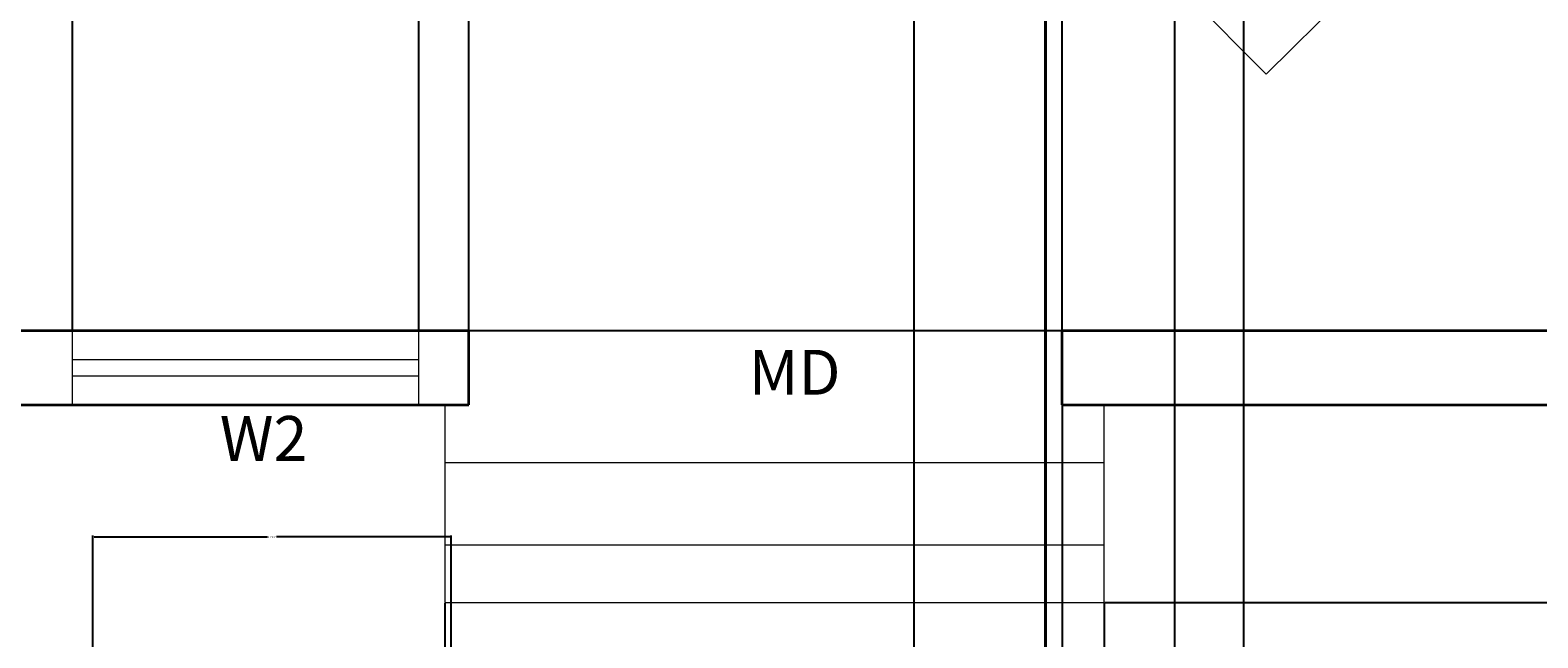
# Model space of a CAD drawing. Units: inches. Extents: x 503 to 1084, y -605 to 132.
# Tile 7 of 14: x 791 to 974, y -392 to -318. Entities that reach past the tile are written whole.
import ezdxf

# ---------------------------------------------------------------- set-up
doc = ezdxf.new("R2010")
doc.units = ezdxf.units.IN
doc.header["$MEASUREMENT"] = 0
for name, color, linetype, lineweight in [('A-ANNO-DIMS', 7, 'Continuous', 18), ('A-ANNO-TEXT', 7, 'Continuous', 18), ('A-FLOR-STRS', 1, 'Continuous', 18), ('wall', 1, 'Continuous', 35), ('wind', 5, 'Continuous', 18)]:
    doc.layers.add(name, color=color, linetype=linetype, lineweight=lineweight)
doc.layers.add('furniture', color=50, linetype='Continuous', lineweight=13, transparency=0.8)
doc.styles.get("Standard").update_dxf_attribs({"font": 'arial.ttf'})
doc.dimstyles.get("Standard").update_dxf_attribs({"dimtxt": 0.18, "dimasz": 0.18, "dimexe": 0.18, "dimexo": 0.0625, "dimgap": 0.09, "dimtad": 0, "dimtih": 1, "dimtoh": 1, "dimdec": 1, "dimzin": 0, "dimdsep": 46, "dimlunit": 4, "dimtxsty": 'Standard', "dimcen": 0.09, "dimadec": 0, "dimazin": 0, "dimtfac": 1, "dimtdec": 1, "dimtofl": 0, "dimtmove": 0, "dimatfit": 3, "dimfxl": 1, "dimtolj": 1, "dimtzin": 0, "dimarcsym": 0})

# ---------------------------------------------------------------- blocks, each defined once
blk = doc.blocks.new('*D37')
at = {"layer": 'A-ANNO-DIMS', "color": 0, "lineweight": -2, "transparency": 16777216}
for p, q in [((798.44, -397.88), (798.44, -379.67)), ((798.62, -379.85), (819.65, -379.85)), ((841.77, -379.85), (820.73, -379.85)), ((841.95, -397.88), (841.95, -379.67))]:
    blk.add_line(p, q, dxfattribs=at)
at = {"layer": 'A-ANNO-DIMS', "color": 0, "transparency": 16777216}
for points in [[(798.62, -379.82), (798.62, -379.88), (798.44, -379.85)], [(841.77, -379.82), (841.77, -379.88), (841.95, -379.85)]]:
    blk.add_solid(points, dxfattribs=at)
at = {"layer": 'Defpoints', "color": 0, "transparency": 16777216}
for p in [(798.44, -379.85), (798.44, -397.95), (841.95, -397.95)]:
    blk.add_point(p, dxfattribs=at)
at = {"layer": 'A-ANNO-DIMS', "color": 0, "transparency": 16777216, "insert": (820.19, -379.85), "char_height": 0.18, "attachment_point": 5}
blk.add_mtext('\\A1;3\'-7 1/2"', dxfattribs=at)
blk = doc.blocks.new('*D45')
at = {"layer": 'A-ANNO-DIMS', "color": 0, "lineweight": -2, "transparency": 16777216}
for p, q in [((844.09, -354.75), (844.09, 43.51)), ((844.27, 43.33), (879.76, 43.33)), ((915.91, 43.33), (880.42, 43.33)), ((916.09, -354.75), (916.09, 43.51))]:
    blk.add_line(p, q, dxfattribs=at)
at = {"layer": 'A-ANNO-DIMS', "color": 0, "transparency": 16777216}
for points in [[(844.27, 43.36), (844.27, 43.3), (844.09, 43.33)], [(915.91, 43.36), (915.91, 43.3), (916.09, 43.33)]]:
    blk.add_solid(points, dxfattribs=at)
at = {"layer": 'Defpoints', "color": 0, "transparency": 16777216}
for p in [(916.09, 43.33), (844.09, -354.82), (916.09, -354.82)]:
    blk.add_point(p, dxfattribs=at)
at = {"layer": 'A-ANNO-DIMS', "color": 0, "transparency": 16777216, "insert": (880.09, 43.33), "char_height": 0.18, "attachment_point": 5}
blk.add_mtext('\\A1;6\'-0"', dxfattribs=at)
blk = doc.blocks.new('*D46')
at = {"layer": 'A-ANNO-DIMS', "color": 0, "lineweight": -2, "transparency": 16777216}
for p, q in [((796, -354.75), (796, 43.51)), ((796.18, 43.33), (816.67, 43.33)), ((837.82, 43.33), (817.33, 43.33)), ((838, -354.75), (838, 43.51))]:
    blk.add_line(p, q, dxfattribs=at)
at = {"layer": 'A-ANNO-DIMS', "color": 0, "transparency": 16777216}
for points in [[(796.18, 43.36), (796.18, 43.3), (796, 43.33)], [(837.82, 43.36), (837.82, 43.3), (838, 43.33)]]:
    blk.add_solid(points, dxfattribs=at)
at = {"layer": 'Defpoints', "color": 0, "transparency": 16777216}
for p in [(838, 43.33), (796, -354.82), (838, -354.82)]:
    blk.add_point(p, dxfattribs=at)
at = {"layer": 'A-ANNO-DIMS', "color": 0, "transparency": 16777216, "insert": (817, 43.33), "char_height": 0.18, "attachment_point": 5}
blk.add_mtext('\\A1;3\'-6"', dxfattribs=at)
blk = doc.blocks.new('*D47')
at = {"layer": 'A-ANNO-DIMS', "color": 0, "lineweight": -2, "transparency": 16777216}
for p, q in [((916.09, -363.88), (916.09, -583.15)), ((986.09, -363.88), (986.09, -583.15)), ((916.27, -582.97), (950.69, -582.97)), ((985.91, -582.97), (951.49, -582.97))]:
    blk.add_line(p, q, dxfattribs=at)
at = {"layer": 'A-ANNO-DIMS', "color": 0, "transparency": 16777216}
for points in [[(916.27, -582.94), (916.27, -583), (916.09, -582.97)], [(985.91, -582.94), (985.91, -583), (986.09, -582.97)]]:
    blk.add_solid(points, dxfattribs=at)
at = {"layer": 'Defpoints', "color": 0, "transparency": 16777216}
for p in [(916.09, -363.82), (986.09, -363.82), (986.09, -582.97)]:
    blk.add_point(p, dxfattribs=at)
at = {"layer": 'A-ANNO-DIMS', "color": 0, "transparency": 16777216, "insert": (951.09, -582.97), "char_height": 0.18, "attachment_point": 5}
blk.add_mtext('\\A1;5\'-10"', dxfattribs=at)
blk = doc.blocks.new('*D48')
at = {"layer": 'A-ANNO-DIMS', "color": 0, "lineweight": -2, "transparency": 16777216}
for p, q in [((783.09, -354.75), (783.09, 43.51)), ((783.27, 43.33), (789.22, 43.33)), ((795.82, 43.33), (789.86, 43.33)), ((796, -354.75), (796, 43.51))]:
    blk.add_line(p, q, dxfattribs=at)
at = {"layer": 'A-ANNO-DIMS', "color": 0, "transparency": 16777216}
for points in [[(783.27, 43.36), (783.27, 43.3), (783.09, 43.33)], [(795.82, 43.36), (795.82, 43.3), (796, 43.33)]]:
    blk.add_solid(points, dxfattribs=at)
at = {"layer": 'Defpoints', "color": 0, "transparency": 16777216}
for p in [(796, 43.33), (783.09, -354.82), (796, -354.82)]:
    blk.add_point(p, dxfattribs=at)
at = {"layer": 'A-ANNO-DIMS', "color": 0, "transparency": 16777216, "insert": (789.54, 43.33), "char_height": 0.18, "attachment_point": 5}
blk.add_mtext('\\A1;1\'-1"', dxfattribs=at)
blk = doc.blocks.new('*D63')
at = {"layer": 'A-ANNO-DIMS', "color": 0, "lineweight": -2, "transparency": 16777216}
for p, q in [((783.15, -281.32), (1083.42, -281.32)), ((1083.24, -281.5), (1083.24, -317.88)), ((1083.24, -354.64), (1083.24, -318.25)), ((783.15, -354.82), (1083.42, -354.82))]:
    blk.add_line(p, q, dxfattribs=at)
at = {"layer": 'A-ANNO-DIMS', "color": 0, "transparency": 16777216}
for points in [[(1083.21, -281.5), (1083.27, -281.5), (1083.24, -281.32)], [(1083.21, -354.64), (1083.27, -354.64), (1083.24, -354.82)]]:
    blk.add_solid(points, dxfattribs=at)
at = {"layer": 'Defpoints', "color": 0, "transparency": 16777216}
for p in [(783.09, -281.32), (783.09, -354.82), (1083.24, -354.82)]:
    blk.add_point(p, dxfattribs=at)
at = {"layer": 'A-ANNO-DIMS', "color": 0, "transparency": 16777216, "insert": (1083.24, -318.07), "char_height": 0.18, "attachment_point": 5}
blk.add_mtext('\\A1;6\'-1 1/2"', dxfattribs=at)
blk = doc.blocks.new('*D64')
at = {"layer": 'A-ANNO-DIMS', "color": 0, "lineweight": -2, "transparency": 16777216}
for p, q in [((938.09, -162.88), (938.09, -583.15)), ((977.09, -162.88), (977.09, -583.15)), ((938.27, -582.97), (957.26, -582.97)), ((976.91, -582.97), (957.92, -582.97))]:
    blk.add_line(p, q, dxfattribs=at)
at = {"layer": 'A-ANNO-DIMS', "color": 0, "transparency": 16777216}
for points in [[(938.27, -582.94), (938.27, -583), (938.09, -582.97)], [(976.91, -582.94), (976.91, -583), (977.09, -582.97)]]:
    blk.add_solid(points, dxfattribs=at)
at = {"layer": 'Defpoints', "color": 0, "transparency": 16777216}
for p in [(938.09, -162.82), (977.09, -162.82), (977.09, -582.97)]:
    blk.add_point(p, dxfattribs=at)
at = {"layer": 'A-ANNO-DIMS', "color": 0, "transparency": 16777216, "insert": (957.59, -582.97), "char_height": 0.18, "attachment_point": 5}
blk.add_mtext('\\A1;3\'-3"', dxfattribs=at)
blk = doc.blocks.new('*D65')
at = {"layer": 'A-ANNO-DIMS', "color": 0, "lineweight": -2, "transparency": 16777216}
for p, q in [((898.09, -162.88), (898.09, -583.15)), ((914.09, -162.88), (914.09, -583.15)), ((898.27, -582.97), (905.77, -582.97)), ((913.91, -582.97), (906.41, -582.97))]:
    blk.add_line(p, q, dxfattribs=at)
at = {"layer": 'A-ANNO-DIMS', "color": 0, "transparency": 16777216}
for points in [[(898.27, -582.94), (898.27, -583), (898.09, -582.97)], [(913.91, -582.94), (913.91, -583), (914.09, -582.97)]]:
    blk.add_solid(points, dxfattribs=at)
at = {"layer": 'Defpoints', "color": 0, "transparency": 16777216}
for p in [(898.09, -162.82), (914.09, -162.82), (914.09, -582.97)]:
    blk.add_point(p, dxfattribs=at)
at = {"layer": 'A-ANNO-DIMS', "color": 0, "transparency": 16777216, "insert": (906.09, -582.97), "char_height": 0.18, "attachment_point": 5}
blk.add_mtext('\\A1;1\'-4"', dxfattribs=at)
blk = doc.blocks.new('*D66')
at = {"layer": 'A-ANNO-DIMS', "color": 0, "lineweight": -2, "transparency": 16777216}
for p, q in [((841.16, -387.88), (841.16, -583.15)), ((921.2, -387.88), (921.2, -583.15)), ((841.34, -582.97), (880.85, -582.97)), ((921.02, -582.97), (881.51, -582.97))]:
    blk.add_line(p, q, dxfattribs=at)
at = {"layer": 'A-ANNO-DIMS', "color": 0, "transparency": 16777216}
for points in [[(841.34, -582.94), (841.34, -583), (841.16, -582.97)], [(921.02, -582.94), (921.02, -583), (921.2, -582.97)]]:
    blk.add_solid(points, dxfattribs=at)
at = {"layer": 'Defpoints', "color": 0, "transparency": 16777216}
for p in [(841.16, -387.82), (921.2, -387.82), (921.2, -582.97)]:
    blk.add_point(p, dxfattribs=at)
at = {"layer": 'A-ANNO-DIMS', "color": 0, "transparency": 16777216, "insert": (881.18, -582.97), "char_height": 0.18, "attachment_point": 5}
blk.add_mtext('\\A1;6\'-8"', dxfattribs=at)
blk = doc.blocks.new('*D67')
at = {"layer": 'A-ANNO-DIMS', "color": 0, "lineweight": -2, "transparency": 16777216}
for p, q in [((921.26, -363.82), (1083.42, -363.82)), ((1083.24, -364), (1083.24, -375.63)), ((1083.24, -387.64), (1083.24, -376)), ((921.26, -387.82), (1083.42, -387.82))]:
    blk.add_line(p, q, dxfattribs=at)
at = {"layer": 'A-ANNO-DIMS', "color": 0, "transparency": 16777216}
for points in [[(1083.21, -364), (1083.27, -364), (1083.24, -363.82)], [(1083.21, -387.64), (1083.27, -387.64), (1083.24, -387.82)]]:
    blk.add_solid(points, dxfattribs=at)
at = {"layer": 'Defpoints', "color": 0, "transparency": 16777216}
for p in [(921.2, -363.82), (1083.24, -363.82), (921.2, -387.82)]:
    blk.add_point(p, dxfattribs=at)
at = {"layer": 'A-ANNO-DIMS', "color": 0, "transparency": 16777216, "insert": (1083.24, -375.82), "char_height": 0.18, "attachment_point": 5}
blk.add_mtext('\\A1;2\'-0"', dxfattribs=at)
blk = doc.blocks.new('*D78')
at = {"layer": 'A-ANNO-DIMS', "color": 0, "lineweight": -2, "transparency": 16777216}
for p, q in [((913.97, -276.31), (913.97, -583.15)), ((929.71, -276.31), (929.71, -583.15)), ((914.15, -582.97), (921.31, -582.97)), ((929.53, -582.97), (922.37, -582.97))]:
    blk.add_line(p, q, dxfattribs=at)
at = {"layer": 'A-ANNO-DIMS', "color": 0, "transparency": 16777216}
for points in [[(914.15, -582.94), (914.15, -583), (913.97, -582.97)], [(929.53, -582.94), (929.53, -583), (929.71, -582.97)]]:
    blk.add_solid(points, dxfattribs=at)
at = {"layer": 'Defpoints', "color": 0, "transparency": 16777216}
for p in [(913.97, -276.25), (929.71, -276.25), (929.71, -582.97)]:
    blk.add_point(p, dxfattribs=at)
at = {"layer": 'A-ANNO-DIMS', "color": 0, "transparency": 16777216, "insert": (921.84, -582.97), "char_height": 0.18, "attachment_point": 5}
blk.add_mtext('\\A1;1\'-3 1/2"', dxfattribs=at)

msp = doc.modelspace()

# ---------------------------------------------------------------- linework, layer by layer
at = {"layer": 'A-FLOR-STRS'}
for p, q in [((841.16, -363.82), (841.16, -387.82)), ((921.2, -387.82), (921.2, -363.82)), ((841.16, -370.82), (921.2, -370.82)), ((841.16, -380.82), (921.2, -380.82)), ((841.16, -387.82), (921.2, -387.82))]:
    msp.add_line(p, q, dxfattribs=at)
at = {"layer": 'furniture'}
for p, q in [((961.01, -303.79), (940.84, -323.7)), ((940.84, -323.7), (923.07, -305.84))]:
    msp.add_line(p, q, dxfattribs=at)
at = {"layer": 'wall'}
for p, q in [((783.09, -354.82), (844.09, -354.82)), ((844.09, -363.82), (844.09, -354.82)), ((916.09, -363.82), (916.09, -354.82)), ((916.09, -354.82), (977.09, -354.82)), ((783.09, -363.82), (844.09, -363.82)), ((916.09, -363.82), (986.09, -363.82))]:
    msp.add_line(p, q, dxfattribs=at)
at = {"layer": 'wind'}
for p, q in [((796, -363.82), (796, -354.82)), ((838, -363.82), (838, -354.82)), ((796, -358.32), (838, -358.32)), ((796, -360.32), (838, -360.32))]:
    msp.add_line(p, q, dxfattribs=at)

# ---------------------------------------------------------------- texts
at = {"layer": 'A-ANNO-TEXT'}
for s, p in [('MD', (878.05, -362.6)), ('W2', (813.86, -370.63))]:
    msp.add_text(s, height=5.444, dxfattribs=at).set_placement(p)

# ---------------------------------------------------------------- dimensions: what is measured, and where the dimension line sits
at = {"layer": 'A-ANNO-DIMS'}
for base, p1, p2, picture, middle in [((796, 43.33), (783.09, -354.82), (796, -354.82), '*D48', (789.54, 43.33)), ((838, 43.33), (796, -354.82), (838, -354.82), '*D46', (817, 43.33)), ((916.09, 43.33), (844.09, -354.82), (916.09, -354.82), '*D45', (880.09, 43.33)), ((914.09, -582.97), (898.09, -162.82), (914.09, -162.82), '*D65', (906.09, -582.97)), ((977.09, -582.97), (938.09, -162.82), (977.09, -162.82), '*D64', (957.59, -582.97)), ((929.71, -582.97), (913.97, -276.25), (929.71, -276.25), '*D78', (921.84, -582.97)), ((986.09, -582.97), (916.09, -363.82), (986.09, -363.82), '*D47', (951.09, -582.97)), ((921.2, -582.97), (841.16, -387.82), (921.2, -387.82), '*D66', (881.18, -582.97))]:
    dim = msp.add_linear_dim(base=base, p1=p1, p2=p2, dimstyle='Standard', override={"dimdec": 1, "dimlfac": 1, "dimrnd": 0, "dimzin": 1, "dimdsep": 46, "dimlunit": 4, "dimfrac": 2}, dxfattribs=at)
    dim.commit()
    dim.dimension.update_dxf_attribs({"geometry": picture, "text_midpoint": middle})
for base, p1, p2, angle, picture, middle in [((1083.24, -354.82), (783.09, -281.32), (783.09, -354.82), 90, '*D63', (1083.24, -318.07)), ((1083.24, -363.82), (921.2, -387.82), (921.2, -363.82), 90, '*D67', (1083.24, -375.82)), ((798.44, -379.85), (841.95, -397.95), (798.44, -397.95), 180, '*D37', (820.19, -379.85))]:
    dim = msp.add_linear_dim(base=base, p1=p1, p2=p2, angle=angle, dimstyle='Standard', override={"dimdec": 1, "dimlfac": 1, "dimrnd": 0, "dimzin": 1, "dimdsep": 46, "dimlunit": 4, "dimfrac": 2}, dxfattribs=at)
    dim.commit()
    dim.dimension.update_dxf_attribs({"geometry": picture, "text_midpoint": middle})

doc.saveas('drawing.dxf')
